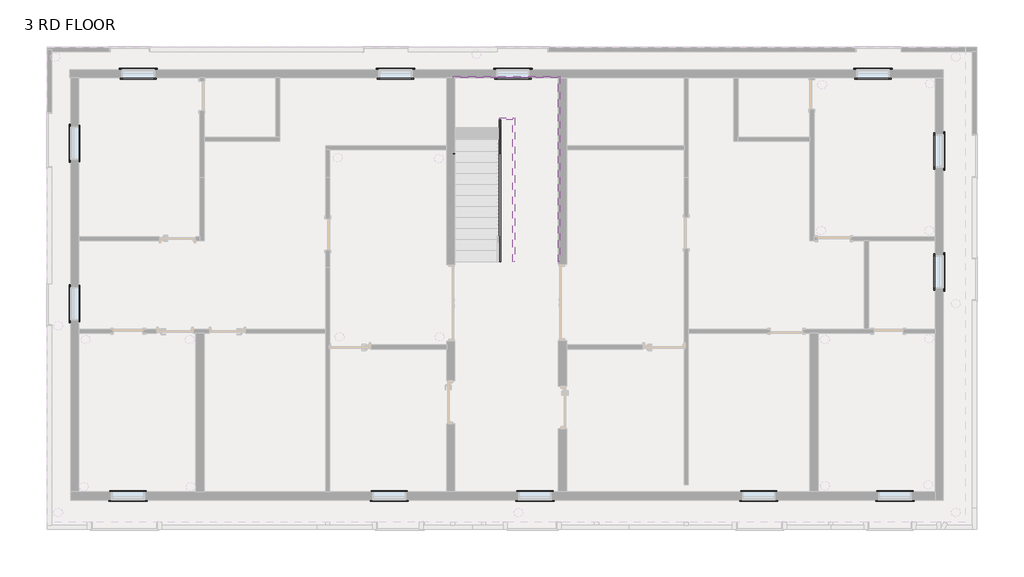
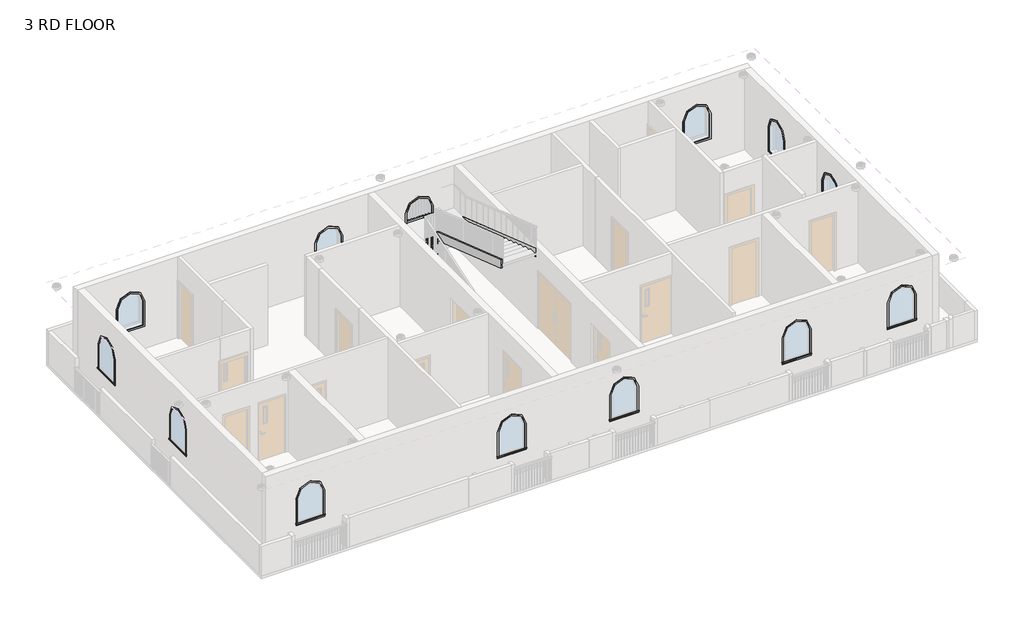
# One storey, part 7 of 7: 26 proxies, 6 members.
"""IFC4 building model written with IfcOpenShell, lengths in millimetres."""

from ifc_helpers import new_model, si_unit, frame, origin, place, context, project, spatial, polyline, outline, extrude, transform, mapped, element, save
from components import trim_window_exterior_flat_arch_top_tree_centered_with_sill_aed3e54d, trim_window_interior_flat_arch_top_tree_centered_picture_e2e46177

model = new_model("IFC4")

# Units and contexts
model_context = context("Model", 3, world=origin())
ifc_project = project(units=[si_unit("LENGTHUNIT", "METRE", prefix="MILLI")], contexts=[model_context])

# Site, building, storey
site = spatial("IfcSite", under=ifc_project)
building = spatial("IfcBuilding", under=site)
storey = spatial("IfcBuildingStorey", under=building, Name="3 RD FLOOR", Elevation=9601.2)

# Proxies
placement = place(None, origin())
trim_window_exterior_flat_arch_top_tree_centered_with_sill_shape = trim_window_exterior_flat_arch_top_tree_centered_with_sill_aed3e54d(model_context)
element("IfcBuildingElementProxy", 1, Name="Trim-Window-Exterior-Flat-Arch-Top-Tree_Centered : with Sill", ObjectType="Trim-Window-Exterior-Flat-Arch-Top-Tree_Centered : with Sill", at=placement, inside=storey, context=model_context, shape_type="MappedRepresentation", body=[
    mapped(trim_window_exterior_flat_arch_top_tree_centered_with_sill_shape, transform((-10865.7987925, -4014.0932193, 11887.2), x_axis=(1.0, 0.0, 0.0), y_axis=(0.0, 0.0, 1.0), z_axis=(0.0, -1.0, 0.0))),
])
element("IfcBuildingElementProxy", 2, Name="Trim-Window-Exterior-Flat-Arch-Top-Tree_Centered : with Sill", ObjectType="Trim-Window-Exterior-Flat-Arch-Top-Tree_Centered : with Sill", at=placement, inside=storey, context=model_context, shape_type="MappedRepresentation", body=[
    mapped(trim_window_exterior_flat_arch_top_tree_centered_with_sill_shape, transform((-3661.7237997, -4014.0932193, 11887.2), x_axis=(1.0, 0.0, 0.0), y_axis=(0.0, 0.0, 1.0), z_axis=(0.0, -1.0, 0.0))),
])
element("IfcBuildingElementProxy", 3, Name="Trim-Window-Exterior-Flat-Arch-Top-Tree_Centered : with Sill", ObjectType="Trim-Window-Exterior-Flat-Arch-Top-Tree_Centered : with Sill", at=placement, inside=storey, context=model_context, shape_type="MappedRepresentation", body=[
    mapped(trim_window_exterior_flat_arch_top_tree_centered_with_sill_shape, transform((360.4932011, -4014.0932193, 11887.2), x_axis=(1.0, 0.0, 0.0), y_axis=(0.0, 0.0, 1.0), z_axis=(0.0, -1.0, 0.0))),
])
element("IfcBuildingElementProxy", 4, Name="Trim-Window-Exterior-Flat-Arch-Top-Tree_Centered : with Sill", ObjectType="Trim-Window-Exterior-Flat-Arch-Top-Tree_Centered : with Sill", at=placement, inside=storey, context=model_context, shape_type="MappedRepresentation", body=[
    mapped(trim_window_exterior_flat_arch_top_tree_centered_with_sill_shape, transform((6533.2012079, -4014.0932193, 11887.2), x_axis=(1.0, 0.0, 0.0), y_axis=(0.0, 0.0, 1.0), z_axis=(0.0, -1.0, 0.0))),
])
element("IfcBuildingElementProxy", 5, Name="Trim-Window-Exterior-Flat-Arch-Top-Tree_Centered : with Sill", ObjectType="Trim-Window-Exterior-Flat-Arch-Top-Tree_Centered : with Sill", at=placement, inside=storey, context=model_context, shape_type="MappedRepresentation", body=[
    mapped(trim_window_exterior_flat_arch_top_tree_centered_with_sill_shape, transform((10292.4012075, -4014.0932193, 11887.2), x_axis=(1.0, 0.0, 0.0), y_axis=(0.0, 0.0, 1.0), z_axis=(0.0, -1.0, 0.0))),
])
element("IfcBuildingElementProxy", 6, Name="Trim-Window-Exterior-Flat-Arch-Top-Tree_Centered : with Sill", ObjectType="Trim-Window-Exterior-Flat-Arch-Top-Tree_Centered : with Sill", at=placement, inside=storey, context=model_context, shape_type="MappedRepresentation", body=[
    mapped(trim_window_exterior_flat_arch_top_tree_centered_with_sill_shape, transform((11625.9012075, 2278.7567332, 11887.2), x_axis=(0.0, 1.0, 0.0), y_axis=(0.0, 0.0, 1.0), z_axis=(1.0, 0.0, 0.0))),
])
element("IfcBuildingElementProxy", 7, Name="Trim-Window-Exterior-Flat-Arch-Top-Tree_Centered : with Sill", ObjectType="Trim-Window-Exterior-Flat-Arch-Top-Tree_Centered : with Sill", at=placement, inside=storey, context=model_context, shape_type="MappedRepresentation", body=[
    mapped(trim_window_exterior_flat_arch_top_tree_centered_with_sill_shape, transform((11625.9012075, 5612.5067329, 11887.2), x_axis=(0.0, 1.0, 0.0), y_axis=(0.0, 0.0, 1.0), z_axis=(1.0, 0.0, 0.0))),
])
element("IfcBuildingElementProxy", 8, Name="Trim-Window-Exterior-Flat-Arch-Top-Tree_Centered : with Sill", ObjectType="Trim-Window-Exterior-Flat-Arch-Top-Tree_Centered : with Sill", at=placement, inside=storey, context=model_context, shape_type="MappedRepresentation", body=[
    mapped(trim_window_exterior_flat_arch_top_tree_centered_with_sill_shape, transform((9682.8012075, 7860.4067329, 11887.2), x_axis=(-1.0, 0.0, 0.0), y_axis=(0.0, 0.0, 1.0), z_axis=(0.0, 1.0, 0.0))),
])
element("IfcBuildingElementProxy", 9, Name="Trim-Window-Exterior-Flat-Arch-Top-Tree_Centered : with Sill", ObjectType="Trim-Window-Exterior-Flat-Arch-Top-Tree_Centered : with Sill", at=placement, inside=storey, context=model_context, shape_type="MappedRepresentation", body=[
    mapped(trim_window_exterior_flat_arch_top_tree_centered_with_sill_shape, transform((-249.1067989, 7860.4067329, 11887.2), x_axis=(-1.0, 0.0, 0.0), y_axis=(0.0, 0.0, 1.0), z_axis=(0.0, 1.0, 0.0))),
])
element("IfcBuildingElementProxy", 10, Name="Trim-Window-Exterior-Flat-Arch-Top-Tree_Centered : with Sill", ObjectType="Trim-Window-Exterior-Flat-Arch-Top-Tree_Centered : with Sill", at=placement, inside=storey, context=model_context, shape_type="MappedRepresentation", body=[
    mapped(trim_window_exterior_flat_arch_top_tree_centered_with_sill_shape, transform((-3487.0987998, 7860.4067329, 11887.2), x_axis=(-1.0, 0.0, 0.0), y_axis=(0.0, 0.0, 1.0), z_axis=(0.0, 1.0, 0.0))),
])
element("IfcBuildingElementProxy", 11, Name="Trim-Window-Exterior-Flat-Arch-Top-Tree_Centered : with Sill", ObjectType="Trim-Window-Exterior-Flat-Arch-Top-Tree_Centered : with Sill", at=placement, inside=storey, context=model_context, shape_type="MappedRepresentation", body=[
    mapped(trim_window_exterior_flat_arch_top_tree_centered_with_sill_shape, transform((-10583.2237959, 7860.4067329, 11887.2), x_axis=(-1.0, 0.0, 0.0), y_axis=(0.0, 0.0, 1.0), z_axis=(0.0, 1.0, 0.0))),
])
element("IfcBuildingElementProxy", 12, Name="Trim-Window-Exterior-Flat-Arch-Top-Tree_Centered : with Sill", ObjectType="Trim-Window-Exterior-Flat-Arch-Top-Tree_Centered : with Sill", at=placement, inside=storey, context=model_context, shape_type="MappedRepresentation", body=[
    mapped(trim_window_exterior_flat_arch_top_tree_centered_with_sill_shape, transform((-12453.2987925, 5825.231733, 11887.2), x_axis=(0.0, -1.0, 0.0), y_axis=(0.0, 0.0, 1.0), z_axis=(-1.0, 0.0, 0.0))),
])
element("IfcBuildingElementProxy", 13, Name="Trim-Window-Exterior-Flat-Arch-Top-Tree_Centered : with Sill", ObjectType="Trim-Window-Exterior-Flat-Arch-Top-Tree_Centered : with Sill", at=placement, inside=storey, context=model_context, shape_type="MappedRepresentation", body=[
    mapped(trim_window_exterior_flat_arch_top_tree_centered_with_sill_shape, transform((-12453.2987925, 1402.4567334, 11887.2), x_axis=(0.0, -1.0, 0.0), y_axis=(0.0, 0.0, 1.0), z_axis=(-1.0, 0.0, 0.0))),
])
trim_window_interior_flat_arch_top_tree_centered_picture_shape = trim_window_interior_flat_arch_top_tree_centered_picture_e2e46177(model_context)
element("IfcBuildingElementProxy", 14, Name="Trim-Window-Interior-Flat-Arch-Top-Tree_Centered : Picture Frame", ObjectType="Trim-Window-Interior-Flat-Arch-Top-Tree_Centered : Picture Frame", at=placement, inside=storey, context=model_context, shape_type="MappedRepresentation", body=[
    mapped(trim_window_interior_flat_arch_top_tree_centered_picture_shape, transform((-10865.7987925, -3785.4932193, 11887.2), x_axis=(-1.0, 0.0, 0.0), y_axis=(0.0, 0.0, 1.0), z_axis=(0.0, 1.0, 0.0))),
])
element("IfcBuildingElementProxy", 15, Name="Trim-Window-Interior-Flat-Arch-Top-Tree_Centered : Picture Frame", ObjectType="Trim-Window-Interior-Flat-Arch-Top-Tree_Centered : Picture Frame", at=placement, inside=storey, context=model_context, shape_type="MappedRepresentation", body=[
    mapped(trim_window_interior_flat_arch_top_tree_centered_picture_shape, transform((-3661.7237997, -3785.4932193, 11887.2), x_axis=(-1.0, 0.0, 0.0), y_axis=(0.0, 0.0, 1.0), z_axis=(0.0, 1.0, 0.0))),
])
element("IfcBuildingElementProxy", 16, Name="Trim-Window-Interior-Flat-Arch-Top-Tree_Centered : Picture Frame", ObjectType="Trim-Window-Interior-Flat-Arch-Top-Tree_Centered : Picture Frame", at=placement, inside=storey, context=model_context, shape_type="MappedRepresentation", body=[
    mapped(trim_window_interior_flat_arch_top_tree_centered_picture_shape, transform((360.4932011, -3785.4932193, 11887.2), x_axis=(-1.0, 0.0, 0.0), y_axis=(0.0, 0.0, 1.0), z_axis=(0.0, 1.0, 0.0))),
])
element("IfcBuildingElementProxy", 17, Name="Trim-Window-Interior-Flat-Arch-Top-Tree_Centered : Picture Frame", ObjectType="Trim-Window-Interior-Flat-Arch-Top-Tree_Centered : Picture Frame", at=placement, inside=storey, context=model_context, shape_type="MappedRepresentation", body=[
    mapped(trim_window_interior_flat_arch_top_tree_centered_picture_shape, transform((6533.2012079, -3785.4932193, 11887.2), x_axis=(-1.0, 0.0, 0.0), y_axis=(0.0, 0.0, 1.0), z_axis=(0.0, 1.0, 0.0))),
])
element("IfcBuildingElementProxy", 18, Name="Trim-Window-Interior-Flat-Arch-Top-Tree_Centered : Picture Frame", ObjectType="Trim-Window-Interior-Flat-Arch-Top-Tree_Centered : Picture Frame", at=placement, inside=storey, context=model_context, shape_type="MappedRepresentation", body=[
    mapped(trim_window_interior_flat_arch_top_tree_centered_picture_shape, transform((10292.4012075, -3785.4932193, 11887.2), x_axis=(-1.0, 0.0, 0.0), y_axis=(0.0, 0.0, 1.0), z_axis=(0.0, 1.0, 0.0))),
])
element("IfcBuildingElementProxy", 19, Name="Trim-Window-Interior-Flat-Arch-Top-Tree_Centered : Picture Frame", ObjectType="Trim-Window-Interior-Flat-Arch-Top-Tree_Centered : Picture Frame", at=placement, inside=storey, context=model_context, shape_type="MappedRepresentation", body=[
    mapped(trim_window_interior_flat_arch_top_tree_centered_picture_shape, transform((11397.3012075, 2278.7567332, 11887.2), x_axis=(0.0, -1.0, 0.0), y_axis=(0.0, 0.0, 1.0), z_axis=(-1.0, 0.0, 0.0))),
])
element("IfcBuildingElementProxy", 20, Name="Trim-Window-Interior-Flat-Arch-Top-Tree_Centered : Picture Frame", ObjectType="Trim-Window-Interior-Flat-Arch-Top-Tree_Centered : Picture Frame", at=placement, inside=storey, context=model_context, shape_type="MappedRepresentation", body=[
    mapped(trim_window_interior_flat_arch_top_tree_centered_picture_shape, transform((11397.3012075, 5612.5067329, 11887.2), x_axis=(0.0, -1.0, 0.0), y_axis=(0.0, 0.0, 1.0), z_axis=(-1.0, 0.0, 0.0))),
])
element("IfcBuildingElementProxy", 21, Name="Trim-Window-Interior-Flat-Arch-Top-Tree_Centered : Picture Frame", ObjectType="Trim-Window-Interior-Flat-Arch-Top-Tree_Centered : Picture Frame", at=placement, inside=storey, context=model_context, shape_type="MappedRepresentation", body=[
    mapped(trim_window_interior_flat_arch_top_tree_centered_picture_shape, transform((9682.8012075, 7631.8067329, 11887.2), x_axis=(1.0, 0.0, 0.0), y_axis=(0.0, 0.0, 1.0), z_axis=(0.0, -1.0, 0.0))),
])
element("IfcBuildingElementProxy", 22, Name="Trim-Window-Interior-Flat-Arch-Top-Tree_Centered : Picture Frame", ObjectType="Trim-Window-Interior-Flat-Arch-Top-Tree_Centered : Picture Frame", at=placement, inside=storey, context=model_context, shape_type="MappedRepresentation", body=[
    mapped(trim_window_interior_flat_arch_top_tree_centered_picture_shape, transform((-249.1067989, 7631.8067329, 11887.2), x_axis=(1.0, 0.0, 0.0), y_axis=(0.0, 0.0, 1.0), z_axis=(0.0, -1.0, 0.0))),
])
element("IfcBuildingElementProxy", 23, Name="Trim-Window-Interior-Flat-Arch-Top-Tree_Centered : Picture Frame", ObjectType="Trim-Window-Interior-Flat-Arch-Top-Tree_Centered : Picture Frame", at=placement, inside=storey, context=model_context, shape_type="MappedRepresentation", body=[
    mapped(trim_window_interior_flat_arch_top_tree_centered_picture_shape, transform((-3487.0987998, 7631.8067329, 11887.2), x_axis=(1.0, 0.0, 0.0), y_axis=(0.0, 0.0, 1.0), z_axis=(0.0, -1.0, 0.0))),
])
element("IfcBuildingElementProxy", 24, Name="Trim-Window-Interior-Flat-Arch-Top-Tree_Centered : Picture Frame", ObjectType="Trim-Window-Interior-Flat-Arch-Top-Tree_Centered : Picture Frame", at=placement, inside=storey, context=model_context, shape_type="MappedRepresentation", body=[
    mapped(trim_window_interior_flat_arch_top_tree_centered_picture_shape, transform((-10583.2237959, 7631.8067329, 11887.2), x_axis=(1.0, 0.0, 0.0), y_axis=(0.0, 0.0, 1.0), z_axis=(0.0, -1.0, 0.0))),
])
element("IfcBuildingElementProxy", 25, Name="Trim-Window-Interior-Flat-Arch-Top-Tree_Centered : Picture Frame", ObjectType="Trim-Window-Interior-Flat-Arch-Top-Tree_Centered : Picture Frame", at=placement, inside=storey, context=model_context, shape_type="MappedRepresentation", body=[
    mapped(trim_window_interior_flat_arch_top_tree_centered_picture_shape, transform((-12224.6987925, 5825.231733, 11887.2), x_axis=(0.0, 1.0, 0.0), y_axis=(0.0, 0.0, 1.0), z_axis=(1.0, 0.0, 0.0))),
])
element("IfcBuildingElementProxy", 26, Name="Trim-Window-Interior-Flat-Arch-Top-Tree_Centered : Picture Frame", ObjectType="Trim-Window-Interior-Flat-Arch-Top-Tree_Centered : Picture Frame", at=placement, inside=storey, context=model_context, shape_type="MappedRepresentation", body=[
    mapped(trim_window_interior_flat_arch_top_tree_centered_picture_shape, transform((-12224.6987925, 1402.4567334, 11887.2), x_axis=(0.0, 1.0, 0.0), y_axis=(0.0, 0.0, 1.0), z_axis=(1.0, 0.0, 0.0))),
])

# Members
element("IfcMember", 27, ObjectType="Stringer - 2\" Width", at=placement, inside=storey, context=model_context, shape_type="SweptSolid", body=[
    extrude(outline(polyline([(2564.5067329, 9601.2), (2564.5067329, 9794.438056), (6486.7524627, 11125.2), (7435.4093802, 11125.2), (2943.6199065, 9601.2), (2564.5067329, 9601.2)])), frame((-1899.5987998, 0.0, 0.0), z_axis=(1.0, 0.0, 0.0), x_axis=(0.0, 1.0, 0.0)), (0.0, 0.0, 1.0), 50.8),
])
element("IfcMember", 28, ObjectType="Stringer - 2\" Width", at=placement, inside=storey, context=model_context, shape_type="SweptSolid", body=[
    extrude(outline(polyline([(-1899.5987998, 7631.8067329), (-1899.5987998, 7682.6067329), (996.0012002, 7682.6067329), (996.0012002, 7631.8067329), (-1899.5987998, 7631.8067329)])), frame((0.0, 0.0, 10820.4), z_axis=(0.0, 0.0, 1.0), x_axis=(1.0, 0.0, 0.0)), (0.0, 0.0, 1.0), 304.8),
])
element("IfcMember", 29, ObjectType="Stringer - 2\" Width", at=placement, inside=storey, context=model_context, shape_type="SweptSolid", body=[
    extrude(outline(polyline([(7682.6067329, 10850.125556), (7682.6067329, 10820.4), (6821.5619804, 10820.4), (2564.5067329, 12264.7580304), (2564.5067329, 12586.6237702), (7682.6067329, 10850.125556)])), frame((996.0012002, 0.0, 0.0), z_axis=(1.0, 0.0, 0.0), x_axis=(0.0, 1.0, 0.0)), (0.0, 0.0, 1.0), 50.8),
])
element("IfcMember", 30, ObjectType="Stringer - 2\" Width", at=placement, inside=storey, context=model_context, shape_type="SweptSolid", body=[
    extrude(outline(polyline([(2564.5067329, 9601.2), (2564.5067329, 9794.438056), (6476.1067329, 11121.588056), (6476.1067329, 10799.7223161), (2943.6199065, 9601.2), (2564.5067329, 9601.2)])), frame((-629.5987998, 0.0, 0.0), z_axis=(1.0, 0.0, 0.0), x_axis=(0.0, 1.0, 0.0)), (0.0, 0.0, 1.0), 50.8),
])
element("IfcMember", 31, ObjectType="Stringer - 2\" Width", at=placement, inside=storey, context=model_context, shape_type="SweptSolid", body=[
    extrude(outline(polyline([(-629.5987998, 6476.1067329), (-629.5987998, 6526.9067329), (-248.5987915, 6526.9067329), (-248.5987915, 6476.1067329), (-629.5987998, 6476.1067329)])), frame((0.0, 0.0, 10820.4), z_axis=(0.0, 0.0, 1.0), x_axis=(1.0, 0.0, 0.0)), (0.0, 0.0, 1.0), 304.8),
])
element("IfcMember", 32, ObjectType="Stringer - 2\" Width", at=placement, inside=storey, context=model_context, shape_type="SweptSolid", body=[
    extrude(outline(polyline([(6526.9067329, 11242.238056), (6526.9067329, 10920.3723161), (2564.5067329, 12264.7580304), (2564.5067329, 12586.6237702), (6526.9067329, 11242.238056)])), frame((-248.5987915, 0.0, 0.0), z_axis=(1.0, 0.0, 0.0), x_axis=(0.0, 1.0, 0.0)), (0.0, 0.0, 1.0), 50.8),
])

save(model, "model.ifc")

# Revit data of these elements
# Type "Trim-Window-Exterior-Flat-Arch-Top-Tree_Centered : with Sill"
#   Trim Width = 0' - 2 1/4"
#   Trim Thickness_Picture Frame = 0' - 1 1/4"
#   Trim Thickness_with Sill = 0' - 0 3/4"
#   Sill Thickness = 0' - 1 1/4"
#   Opening Width [instance default] = 2' - 0"
#   Opening Height [instance default] = 3' - 0"
#   Default Elevation = 4' - 0"
#   Sill = yes
#   Picture Frame = no
#   Trim Material [instance default] = none
# Type "Trim-Window-Interior-Flat-Arch-Top-Tree_Centered : Picture Frame"
#   Trim Thickness_Picture Frame = 0' - 1 1/4"
#   Trim Width = 0' - 2 1/4"
#   Trim Thickness_with Sill = 0' - 0 3/4"
#   Sill Thickness = 0' - 1 1/4"
#   Opening Width [instance default] = 2' - 0"
#   Opening Height [instance default] = 3' - 0"
#   Default Elevation = 4' - 0"
#   Sill = no
#   Picture Frame = yes
#   Trim Material [instance default] = none
# Elements 1, 2, 3, 4, 5, 6, 7, 8, 9, 10, 11, 12, 13 (IfcBuildingElementProxy, "Trim-Window-Exterior-Flat-Arch-Top-Tree_Centered : with Sill")
#   Opening Width = 3' - 0"
#   Opening Height = 4' - 6"
#   Trim Material = Clad - White
#   Phase Created = New Construction
#   Materials on its faces: "Clad - White"
# Elements 14, 15, 16, 17, 18, 19, 20, 21, 22, 23, 24, 25, 26 (IfcBuildingElementProxy, "Trim-Window-Interior-Flat-Arch-Top-Tree_Centered : Picture Frame")
#   Opening Width = 3' - 0"
#   Opening Height = 4' - 6"
#   Trim Material = Wood - Stained
#   Phase Created = New Construction
#   Materials on its faces: "Wood - Stained"
# Elements 27, 28, 29, 30, 31, 32 (IfcMember, "Stringer - 2\" Width")
#   Phase Created = New Construction
# Materials
#   "Clad - White": class "Wood", colour RGB 242 242 238, transparency 0, Cost = 0
#   "Wood - Stained": class "Wood", colour RGB 224 178 126, transparency 0, Cost = 0
